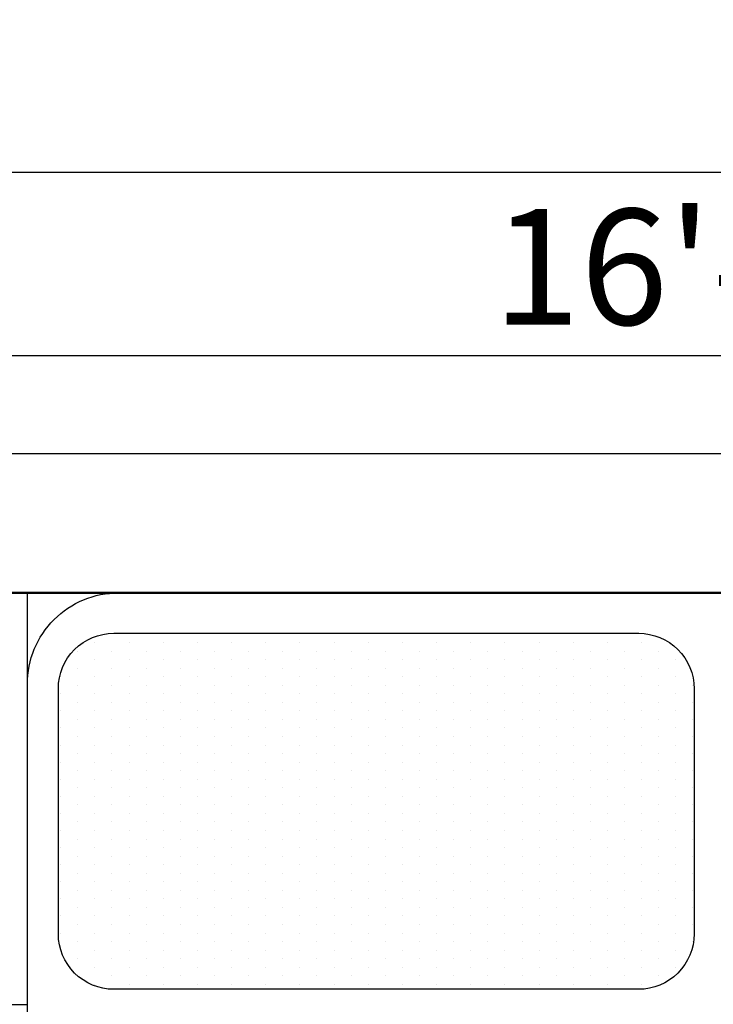
# Model space of a CAD drawing. Units: inches. Extents: x 3064 to 19385, y 846 to 15425.
# Tile 32 of 108: x 4973 to 5003, y 1368 to 1411. Entities that reach past the tile are written whole.
import ezdxf

# ---------------------------------------------------------------- set-up
doc = ezdxf.new("R2010")
doc.units = ezdxf.units.IN
for name, color, linetype, lineweight in [('A-ANNO-DIMS', 2, 'Continuous', 18), ('A-FLOR-FIXT', 9, 'Continuous', 18), ('A-WALL', 7, 'Continuous', 50), ('C-PROP', 6, 'Continuous', 25)]:
    doc.layers.add(name, color=color, linetype=linetype, lineweight=lineweight)
doc.layers.add('BLOCK', color=6, linetype='Continuous')
doc.styles.get("Standard").update_dxf_attribs({"font": 'arial.ttf'})
doc.dimstyles.new('ISO-25', dxfattribs={"dimtxt": 9, "dimasz": 2.5, "dimexe": 1.25, "dimexo": 0.625, "dimtad": 1, "dimdec": 1, "dimlunit": 3, "dimtxsty": 'Standard', "dimcen": 2.5, "dimadec": 0, "dimazin": 0, "dimtfac": 1, "dimtdec": 1, "dimtmove": 0, "dimatfit": 3, "dimfxl": 1, "dimarcsym": 0})

# ---------------------------------------------------------------- blocks, each defined once
blk = doc.blocks.new('*X7')
at = {"color": 0}
for p, q in [((266.25, 456.9375), (266.25, 456.9375)), ((266.4375, 457.03125), (266.4375, 457.03125)), ((266.625, 456.9375), (266.625, 456.9375)), ((266.8125, 457.03125), (266.8125, 457.03125)), ((267, 456.9375), (267, 456.9375)), ((267.1875, 457.03125), (267.1875, 457.03125)), ((267.375, 456.9375), (267.375, 456.9375)), ((267.5625, 457.03125), (267.5625, 457.03125)), ((267.75, 456.9375), (267.75, 456.9375)), ((267.9375, 457.03125), (267.9375, 457.03125)), ((268.125, 456.9375), (268.125, 456.9375)), ((268.3125, 457.03125), (268.3125, 457.03125)), ((268.5, 456.9375), (268.5, 456.9375)), ((268.6875, 457.03125), (268.6875, 457.03125)), ((268.875, 456.9375), (268.875, 456.9375)), ((269.0625, 457.03125), (269.0625, 457.03125)), ((269.25, 456.9375), (269.25, 456.9375)), ((269.4375, 457.03125), (269.4375, 457.03125)), ((269.625, 456.9375), (269.625, 456.9375)), ((269.8125, 457.03125), (269.8125, 457.03125)), ((270, 456.9375), (270, 456.9375)), ((270.1875, 457.03125), (270.1875, 457.03125)), ((270.375, 456.9375), (270.375, 456.9375)), ((270.5625, 457.03125), (270.5625, 457.03125)), ((270.75, 456.9375), (270.75, 456.9375)), ((270.9375, 457.03125), (270.9375, 457.03125)), ((271.125, 456.9375), (271.125, 456.9375)), ((271.3125, 457.03125), (271.3125, 457.03125)), ((271.5, 456.9375), (271.5, 456.9375)), ((271.6875, 457.03125), (271.6875, 457.03125)), ((271.875, 456.9375), (271.875, 456.9375)), ((272.0625, 457.03125), (272.0625, 457.03125)), ((272.25, 456.9375), (272.25, 456.9375)), ((266.0625, 456.84375), (266.0625, 456.84375)), ((266.4375, 456.84375), (266.4375, 456.84375)), ((266.8125, 456.84375), (266.8125, 456.84375)), ((267.1875, 456.84375), (267.1875, 456.84375)), ((267.5625, 456.84375), (267.5625, 456.84375)), ((267.9375, 456.84375), (267.9375, 456.84375)), ((268.3125, 456.84375), (268.3125, 456.84375)), ((268.6875, 456.84375), (268.6875, 456.84375)), ((269.0625, 456.84375), (269.0625, 456.84375)), ((269.4375, 456.84375), (269.4375, 456.84375)), ((269.8125, 456.84375), (269.8125, 456.84375)), ((270.1875, 456.84375), (270.1875, 456.84375)), ((270.5625, 456.84375), (270.5625, 456.84375)), ((270.9375, 456.84375), (270.9375, 456.84375)), ((271.3125, 456.84375), (271.3125, 456.84375)), ((271.6875, 456.84375), (271.6875, 456.84375)), ((272.0625, 456.84375), (272.0625, 456.84375)), ((272.4375, 456.84375), (272.4375, 456.84375)), ((266.25, 456.75), (266.25, 456.75)), ((266.625, 456.75), (266.625, 456.75)), ((267, 456.75), (267, 456.75)), ((267.375, 456.75), (267.375, 456.75)), ((267.75, 456.75), (267.75, 456.75)), ((268.125, 456.75), (268.125, 456.75)), ((268.5, 456.75), (268.5, 456.75)), ((268.875, 456.75), (268.875, 456.75)), ((269.25, 456.75), (269.25, 456.75)), ((269.625, 456.75), (269.625, 456.75)), ((270, 456.75), (270, 456.75)), ((270.375, 456.75), (270.375, 456.75)), ((270.75, 456.75), (270.75, 456.75)), ((271.125, 456.75), (271.125, 456.75)), ((271.5, 456.75), (271.5, 456.75)), ((271.875, 456.75), (271.875, 456.75)), ((272.25, 456.75), (272.25, 456.75)), ((272.625, 456.75), (272.625, 456.75)), ((266.0625, 456.65625), (266.0625, 456.65625)), ((266.4375, 456.65625), (266.4375, 456.65625)), ((266.8125, 456.65625), (266.8125, 456.65625)), ((267.1875, 456.65625), (267.1875, 456.65625)), ((267.5625, 456.65625), (267.5625, 456.65625)), ((267.9375, 456.65625), (267.9375, 456.65625)), ((268.3125, 456.65625), (268.3125, 456.65625)), ((268.6875, 456.65625), (268.6875, 456.65625)), ((269.0625, 456.65625), (269.0625, 456.65625)), ((269.4375, 456.65625), (269.4375, 456.65625)), ((269.8125, 456.65625), (269.8125, 456.65625)), ((270.1875, 456.65625), (270.1875, 456.65625)), ((270.5625, 456.65625), (270.5625, 456.65625)), ((270.9375, 456.65625), (270.9375, 456.65625)), ((271.3125, 456.65625), (271.3125, 456.65625)), ((271.6875, 456.65625), (271.6875, 456.65625)), ((272.0625, 456.65625), (272.0625, 456.65625)), ((272.4375, 456.65625), (272.4375, 456.65625)), ((265.875, 456.5625), (265.875, 456.5625)), ((266.25, 456.5625), (266.25, 456.5625)), ((266.625, 456.5625), (266.625, 456.5625)), ((267, 456.5625), (267, 456.5625)), ((267.375, 456.5625), (267.375, 456.5625)), ((267.75, 456.5625), (267.75, 456.5625)), ((268.125, 456.5625), (268.125, 456.5625)), ((268.5, 456.5625), (268.5, 456.5625)), ((268.875, 456.5625), (268.875, 456.5625)), ((269.25, 456.5625), (269.25, 456.5625)), ((269.625, 456.5625), (269.625, 456.5625)), ((270, 456.5625), (270, 456.5625)), ((270.375, 456.5625), (270.375, 456.5625)), ((270.75, 456.5625), (270.75, 456.5625)), ((271.125, 456.5625), (271.125, 456.5625)), ((271.5, 456.5625), (271.5, 456.5625)), ((271.875, 456.5625), (271.875, 456.5625)), ((272.25, 456.5625), (272.25, 456.5625)), ((272.625, 456.5625), (272.625, 456.5625)), ((266.0625, 456.46875), (266.0625, 456.46875)), ((266.4375, 456.46875), (266.4375, 456.46875)), ((266.8125, 456.46875), (266.8125, 456.46875)), ((267.1875, 456.46875), (267.1875, 456.46875)), ((267.5625, 456.46875), (267.5625, 456.46875)), ((267.9375, 456.46875), (267.9375, 456.46875)), ((268.3125, 456.46875), (268.3125, 456.46875)), ((268.6875, 456.46875), (268.6875, 456.46875)), ((269.0625, 456.46875), (269.0625, 456.46875)), ((269.4375, 456.46875), (269.4375, 456.46875)), ((269.8125, 456.46875), (269.8125, 456.46875)), ((270.1875, 456.46875), (270.1875, 456.46875)), ((270.5625, 456.46875), (270.5625, 456.46875)), ((270.9375, 456.46875), (270.9375, 456.46875)), ((271.3125, 456.46875), (271.3125, 456.46875)), ((271.6875, 456.46875), (271.6875, 456.46875)), ((272.0625, 456.46875), (272.0625, 456.46875)), ((272.4375, 456.46875), (272.4375, 456.46875)), ((272.8125, 456.46875), (272.8125, 456.46875)), ((265.875, 456.375), (265.875, 456.375)), ((266.25, 456.375), (266.25, 456.375)), ((266.625, 456.375), (266.625, 456.375)), ((267, 456.375), (267, 456.375)), ((267.375, 456.375), (267.375, 456.375)), ((267.75, 456.375), (267.75, 456.375)), ((268.125, 456.375), (268.125, 456.375)), ((268.5, 456.375), (268.5, 456.375)), ((268.875, 456.375), (268.875, 456.375)), ((269.25, 456.375), (269.25, 456.375)), ((269.625, 456.375), (269.625, 456.375)), ((270, 456.375), (270, 456.375)), ((270.375, 456.375), (270.375, 456.375)), ((270.75, 456.375), (270.75, 456.375)), ((271.125, 456.375), (271.125, 456.375)), ((271.5, 456.375), (271.5, 456.375)), ((271.875, 456.375), (271.875, 456.375)), ((272.25, 456.375), (272.25, 456.375)), ((272.625, 456.375), (272.625, 456.375)), ((265.875, 456.1875), (265.875, 456.1875)), ((266.0625, 456.28125), (266.0625, 456.28125)), ((266.25, 456.1875), (266.25, 456.1875)), ((266.4375, 456.28125), (266.4375, 456.28125)), ((266.625, 456.1875), (266.625, 456.1875)), ((266.8125, 456.28125), (266.8125, 456.28125)), ((267, 456.1875), (267, 456.1875)), ((267.1875, 456.28125), (267.1875, 456.28125)), ((267.375, 456.1875), (267.375, 456.1875)), ((267.5625, 456.28125), (267.5625, 456.28125)), ((267.75, 456.1875), (267.75, 456.1875)), ((267.9375, 456.28125), (267.9375, 456.28125)), ((268.125, 456.1875), (268.125, 456.1875)), ((268.3125, 456.28125), (268.3125, 456.28125)), ((268.5, 456.1875), (268.5, 456.1875)), ((268.6875, 456.28125), (268.6875, 456.28125)), ((268.875, 456.1875), (268.875, 456.1875)), ((269.0625, 456.28125), (269.0625, 456.28125)), ((269.25, 456.1875), (269.25, 456.1875)), ((269.4375, 456.28125), (269.4375, 456.28125)), ((269.625, 456.1875), (269.625, 456.1875)), ((269.8125, 456.28125), (269.8125, 456.28125)), ((270, 456.1875), (270, 456.1875)), ((270.1875, 456.28125), (270.1875, 456.28125)), ((270.375, 456.1875), (270.375, 456.1875)), ((270.5625, 456.28125), (270.5625, 456.28125)), ((270.75, 456.1875), (270.75, 456.1875)), ((270.9375, 456.28125), (270.9375, 456.28125)), ((271.125, 456.1875), (271.125, 456.1875)), ((271.3125, 456.28125), (271.3125, 456.28125)), ((271.5, 456.1875), (271.5, 456.1875)), ((271.6875, 456.28125), (271.6875, 456.28125)), ((271.875, 456.1875), (271.875, 456.1875)), ((272.0625, 456.28125), (272.0625, 456.28125)), ((272.25, 456.1875), (272.25, 456.1875)), ((272.4375, 456.28125), (272.4375, 456.28125)), ((272.625, 456.1875), (272.625, 456.1875)), ((272.8125, 456.28125), (272.8125, 456.28125)), ((266.0625, 456.09375), (266.0625, 456.09375)), ((266.4375, 456.09375), (266.4375, 456.09375)), ((266.8125, 456.09375), (266.8125, 456.09375)), ((267.1875, 456.09375), (267.1875, 456.09375)), ((267.5625, 456.09375), (267.5625, 456.09375)), ((267.9375, 456.09375), (267.9375, 456.09375)), ((268.3125, 456.09375), (268.3125, 456.09375)), ((268.6875, 456.09375), (268.6875, 456.09375)), ((269.0625, 456.09375), (269.0625, 456.09375)), ((269.4375, 456.09375), (269.4375, 456.09375)), ((269.8125, 456.09375), (269.8125, 456.09375)), ((270.1875, 456.09375), (270.1875, 456.09375)), ((270.5625, 456.09375), (270.5625, 456.09375)), ((270.9375, 456.09375), (270.9375, 456.09375)), ((271.3125, 456.09375), (271.3125, 456.09375)), ((271.6875, 456.09375), (271.6875, 456.09375)), ((272.0625, 456.09375), (272.0625, 456.09375)), ((272.4375, 456.09375), (272.4375, 456.09375)), ((272.8125, 456.09375), (272.8125, 456.09375)), ((265.875, 456), (265.875, 456)), ((266.25, 456), (266.25, 456)), ((266.625, 456), (266.625, 456)), ((267, 456), (267, 456)), ((267.375, 456), (267.375, 456)), ((267.75, 456), (267.75, 456)), ((268.125, 456), (268.125, 456)), ((268.5, 456), (268.5, 456)), ((268.875, 456), (268.875, 456)), ((269.25, 456), (269.25, 456)), ((269.625, 456), (269.625, 456)), ((270, 456), (270, 456)), ((270.375, 456), (270.375, 456)), ((270.75, 456), (270.75, 456)), ((271.125, 456), (271.125, 456)), ((271.5, 456), (271.5, 456)), ((271.875, 456), (271.875, 456)), ((272.25, 456), (272.25, 456)), ((272.625, 456), (272.625, 456)), ((266.0625, 455.90625), (266.0625, 455.90625)), ((266.4375, 455.90625), (266.4375, 455.90625)), ((266.8125, 455.90625), (266.8125, 455.90625)), ((267.1875, 455.90625), (267.1875, 455.90625)), ((267.5625, 455.90625), (267.5625, 455.90625)), ((267.9375, 455.90625), (267.9375, 455.90625)), ((268.3125, 455.90625), (268.3125, 455.90625)), ((268.6875, 455.90625), (268.6875, 455.90625)), ((269.0625, 455.90625), (269.0625, 455.90625)), ((269.4375, 455.90625), (269.4375, 455.90625)), ((269.8125, 455.90625), (269.8125, 455.90625)), ((270.1875, 455.90625), (270.1875, 455.90625)), ((270.5625, 455.90625), (270.5625, 455.90625)), ((270.9375, 455.90625), (270.9375, 455.90625)), ((271.3125, 455.90625), (271.3125, 455.90625)), ((271.6875, 455.90625), (271.6875, 455.90625)), ((272.0625, 455.90625), (272.0625, 455.90625)), ((272.4375, 455.90625), (272.4375, 455.90625)), ((272.8125, 455.90625), (272.8125, 455.90625)), ((265.875, 455.8125), (265.875, 455.8125)), ((266.25, 455.8125), (266.25, 455.8125)), ((266.625, 455.8125), (266.625, 455.8125)), ((267, 455.8125), (267, 455.8125)), ((267.375, 455.8125), (267.375, 455.8125)), ((267.75, 455.8125), (267.75, 455.8125)), ((268.125, 455.8125), (268.125, 455.8125)), ((268.5, 455.8125), (268.5, 455.8125)), ((268.875, 455.8125), (268.875, 455.8125)), ((269.25, 455.8125), (269.25, 455.8125)), ((269.625, 455.8125), (269.625, 455.8125)), ((270, 455.8125), (270, 455.8125)), ((270.375, 455.8125), (270.375, 455.8125)), ((270.75, 455.8125), (270.75, 455.8125)), ((271.125, 455.8125), (271.125, 455.8125)), ((271.5, 455.8125), (271.5, 455.8125)), ((271.875, 455.8125), (271.875, 455.8125)), ((272.25, 455.8125), (272.25, 455.8125)), ((272.625, 455.8125), (272.625, 455.8125)), ((266.0625, 455.71875), (266.0625, 455.71875)), ((266.4375, 455.71875), (266.4375, 455.71875)), ((266.8125, 455.71875), (266.8125, 455.71875)), ((267.1875, 455.71875), (267.1875, 455.71875)), ((267.5625, 455.71875), (267.5625, 455.71875)), ((267.9375, 455.71875), (267.9375, 455.71875)), ((268.3125, 455.71875), (268.3125, 455.71875)), ((268.6875, 455.71875), (268.6875, 455.71875)), ((269.0625, 455.71875), (269.0625, 455.71875)), ((269.4375, 455.71875), (269.4375, 455.71875)), ((269.8125, 455.71875), (269.8125, 455.71875)), ((270.1875, 455.71875), (270.1875, 455.71875)), ((270.5625, 455.71875), (270.5625, 455.71875)), ((270.9375, 455.71875), (270.9375, 455.71875)), ((271.3125, 455.71875), (271.3125, 455.71875)), ((271.6875, 455.71875), (271.6875, 455.71875)), ((272.0625, 455.71875), (272.0625, 455.71875)), ((272.4375, 455.71875), (272.4375, 455.71875)), ((272.8125, 455.71875), (272.8125, 455.71875)), ((265.875, 455.625), (265.875, 455.625)), ((266.0625, 455.53125), (266.0625, 455.53125)), ((266.25, 455.625), (266.25, 455.625)), ((266.4375, 455.53125), (266.4375, 455.53125)), ((266.625, 455.625), (266.625, 455.625)), ((266.8125, 455.53125), (266.8125, 455.53125)), ((267, 455.625), (267, 455.625)), ((267.1875, 455.53125), (267.1875, 455.53125)), ((267.375, 455.625), (267.375, 455.625)), ((267.5625, 455.53125), (267.5625, 455.53125)), ((267.75, 455.625), (267.75, 455.625)), ((267.9375, 455.53125), (267.9375, 455.53125)), ((268.125, 455.625), (268.125, 455.625)), ((268.3125, 455.53125), (268.3125, 455.53125)), ((268.5, 455.625), (268.5, 455.625)), ((268.6875, 455.53125), (268.6875, 455.53125)), ((268.875, 455.625), (268.875, 455.625)), ((269.0625, 455.53125), (269.0625, 455.53125)), ((269.25, 455.625), (269.25, 455.625)), ((269.4375, 455.53125), (269.4375, 455.53125)), ((269.625, 455.625), (269.625, 455.625)), ((269.8125, 455.53125), (269.8125, 455.53125)), ((270, 455.625), (270, 455.625)), ((270.1875, 455.53125), (270.1875, 455.53125)), ((270.375, 455.625), (270.375, 455.625)), ((270.5625, 455.53125), (270.5625, 455.53125)), ((270.75, 455.625), (270.75, 455.625)), ((270.9375, 455.53125), (270.9375, 455.53125)), ((271.125, 455.625), (271.125, 455.625)), ((271.3125, 455.53125), (271.3125, 455.53125)), ((271.5, 455.625), (271.5, 455.625)), ((271.6875, 455.53125), (271.6875, 455.53125)), ((271.875, 455.625), (271.875, 455.625)), ((272.0625, 455.53125), (272.0625, 455.53125)), ((272.25, 455.625), (272.25, 455.625)), ((272.4375, 455.53125), (272.4375, 455.53125)), ((272.625, 455.625), (272.625, 455.625)), ((272.8125, 455.53125), (272.8125, 455.53125)), ((265.875, 455.4375), (265.875, 455.4375)), ((266.25, 455.4375), (266.25, 455.4375)), ((266.625, 455.4375), (266.625, 455.4375)), ((267, 455.4375), (267, 455.4375)), ((267.375, 455.4375), (267.375, 455.4375)), ((267.75, 455.4375), (267.75, 455.4375)), ((268.125, 455.4375), (268.125, 455.4375)), ((268.5, 455.4375), (268.5, 455.4375)), ((268.875, 455.4375), (268.875, 455.4375)), ((269.25, 455.4375), (269.25, 455.4375)), ((269.625, 455.4375), (269.625, 455.4375)), ((270, 455.4375), (270, 455.4375)), ((270.375, 455.4375), (270.375, 455.4375)), ((270.75, 455.4375), (270.75, 455.4375)), ((271.125, 455.4375), (271.125, 455.4375)), ((271.5, 455.4375), (271.5, 455.4375)), ((271.875, 455.4375), (271.875, 455.4375)), ((272.25, 455.4375), (272.25, 455.4375)), ((272.625, 455.4375), (272.625, 455.4375)), ((266.0625, 455.34375), (266.0625, 455.34375)), ((266.4375, 455.34375), (266.4375, 455.34375)), ((266.8125, 455.34375), (266.8125, 455.34375)), ((267.1875, 455.34375), (267.1875, 455.34375)), ((267.5625, 455.34375), (267.5625, 455.34375)), ((267.9375, 455.34375), (267.9375, 455.34375)), ((268.3125, 455.34375), (268.3125, 455.34375)), ((268.6875, 455.34375), (268.6875, 455.34375)), ((269.0625, 455.34375), (269.0625, 455.34375)), ((269.4375, 455.34375), (269.4375, 455.34375)), ((269.8125, 455.34375), (269.8125, 455.34375)), ((270.1875, 455.34375), (270.1875, 455.34375)), ((270.5625, 455.34375), (270.5625, 455.34375)), ((270.9375, 455.34375), (270.9375, 455.34375)), ((271.3125, 455.34375), (271.3125, 455.34375)), ((271.6875, 455.34375), (271.6875, 455.34375)), ((272.0625, 455.34375), (272.0625, 455.34375)), ((272.4375, 455.34375), (272.4375, 455.34375)), ((272.8125, 455.34375), (272.8125, 455.34375)), ((265.875, 455.25), (265.875, 455.25)), ((266.25, 455.25), (266.25, 455.25)), ((266.625, 455.25), (266.625, 455.25)), ((267, 455.25), (267, 455.25)), ((267.375, 455.25), (267.375, 455.25)), ((267.75, 455.25), (267.75, 455.25)), ((268.125, 455.25), (268.125, 455.25)), ((268.5, 455.25), (268.5, 455.25)), ((268.875, 455.25), (268.875, 455.25)), ((269.25, 455.25), (269.25, 455.25)), ((269.625, 455.25), (269.625, 455.25)), ((270, 455.25), (270, 455.25)), ((270.375, 455.25), (270.375, 455.25)), ((270.75, 455.25), (270.75, 455.25)), ((271.125, 455.25), (271.125, 455.25)), ((271.5, 455.25), (271.5, 455.25)), ((271.875, 455.25), (271.875, 455.25)), ((272.25, 455.25), (272.25, 455.25)), ((272.625, 455.25), (272.625, 455.25)), ((266.0625, 455.15625), (266.0625, 455.15625)), ((266.4375, 455.15625), (266.4375, 455.15625)), ((266.8125, 455.15625), (266.8125, 455.15625)), ((267.1875, 455.15625), (267.1875, 455.15625)), ((267.5625, 455.15625), (267.5625, 455.15625)), ((267.9375, 455.15625), (267.9375, 455.15625)), ((268.3125, 455.15625), (268.3125, 455.15625)), ((268.6875, 455.15625), (268.6875, 455.15625)), ((269.0625, 455.15625), (269.0625, 455.15625)), ((269.4375, 455.15625), (269.4375, 455.15625)), ((269.8125, 455.15625), (269.8125, 455.15625)), ((270.1875, 455.15625), (270.1875, 455.15625)), ((270.5625, 455.15625), (270.5625, 455.15625)), ((270.9375, 455.15625), (270.9375, 455.15625)), ((271.3125, 455.15625), (271.3125, 455.15625)), ((271.6875, 455.15625), (271.6875, 455.15625)), ((272.0625, 455.15625), (272.0625, 455.15625)), ((272.4375, 455.15625), (272.4375, 455.15625)), ((272.8125, 455.15625), (272.8125, 455.15625)), ((265.875, 455.0625), (265.875, 455.0625)), ((266.25, 455.0625), (266.25, 455.0625)), ((266.625, 455.0625), (266.625, 455.0625)), ((267, 455.0625), (267, 455.0625)), ((267.375, 455.0625), (267.375, 455.0625)), ((267.75, 455.0625), (267.75, 455.0625)), ((268.125, 455.0625), (268.125, 455.0625)), ((268.5, 455.0625), (268.5, 455.0625)), ((268.875, 455.0625), (268.875, 455.0625)), ((269.25, 455.0625), (269.25, 455.0625)), ((269.625, 455.0625), (269.625, 455.0625)), ((270, 455.0625), (270, 455.0625)), ((270.375, 455.0625), (270.375, 455.0625)), ((270.75, 455.0625), (270.75, 455.0625)), ((271.125, 455.0625), (271.125, 455.0625)), ((271.5, 455.0625), (271.5, 455.0625)), ((271.875, 455.0625), (271.875, 455.0625)), ((272.25, 455.0625), (272.25, 455.0625)), ((272.625, 455.0625), (272.625, 455.0625)), ((266.0625, 454.96875), (266.0625, 454.96875)), ((266.4375, 454.96875), (266.4375, 454.96875)), ((266.8125, 454.96875), (266.8125, 454.96875)), ((267.1875, 454.96875), (267.1875, 454.96875)), ((267.5625, 454.96875), (267.5625, 454.96875)), ((267.9375, 454.96875), (267.9375, 454.96875)), ((268.3125, 454.96875), (268.3125, 454.96875)), ((268.6875, 454.96875), (268.6875, 454.96875)), ((269.0625, 454.96875), (269.0625, 454.96875)), ((269.4375, 454.96875), (269.4375, 454.96875)), ((269.8125, 454.96875), (269.8125, 454.96875)), ((270.1875, 454.96875), (270.1875, 454.96875)), ((270.5625, 454.96875), (270.5625, 454.96875)), ((270.9375, 454.96875), (270.9375, 454.96875)), ((271.3125, 454.96875), (271.3125, 454.96875)), ((271.6875, 454.96875), (271.6875, 454.96875)), ((272.0625, 454.96875), (272.0625, 454.96875)), ((272.4375, 454.96875), (272.4375, 454.96875)), ((272.8125, 454.96875), (272.8125, 454.96875)), ((265.875, 454.875), (265.875, 454.875)), ((266.0625, 454.78125), (266.0625, 454.78125)), ((266.25, 454.875), (266.25, 454.875)), ((266.4375, 454.78125), (266.4375, 454.78125)), ((266.625, 454.875), (266.625, 454.875)), ((266.8125, 454.78125), (266.8125, 454.78125)), ((267, 454.875), (267, 454.875)), ((267.1875, 454.78125), (267.1875, 454.78125)), ((267.375, 454.875), (267.375, 454.875)), ((267.5625, 454.78125), (267.5625, 454.78125)), ((267.75, 454.875), (267.75, 454.875)), ((267.9375, 454.78125), (267.9375, 454.78125)), ((268.125, 454.875), (268.125, 454.875)), ((268.3125, 454.78125), (268.3125, 454.78125)), ((268.5, 454.875), (268.5, 454.875)), ((268.6875, 454.78125), (268.6875, 454.78125)), ((268.875, 454.875), (268.875, 454.875)), ((269.0625, 454.78125), (269.0625, 454.78125)), ((269.25, 454.875), (269.25, 454.875)), ((269.4375, 454.78125), (269.4375, 454.78125)), ((269.625, 454.875), (269.625, 454.875)), ((269.8125, 454.78125), (269.8125, 454.78125)), ((270, 454.875), (270, 454.875)), ((270.1875, 454.78125), (270.1875, 454.78125)), ((270.375, 454.875), (270.375, 454.875)), ((270.5625, 454.78125), (270.5625, 454.78125)), ((270.75, 454.875), (270.75, 454.875)), ((270.9375, 454.78125), (270.9375, 454.78125)), ((271.125, 454.875), (271.125, 454.875)), ((271.3125, 454.78125), (271.3125, 454.78125)), ((271.5, 454.875), (271.5, 454.875)), ((271.6875, 454.78125), (271.6875, 454.78125)), ((271.875, 454.875), (271.875, 454.875)), ((272.0625, 454.78125), (272.0625, 454.78125)), ((272.25, 454.875), (272.25, 454.875)), ((272.4375, 454.78125), (272.4375, 454.78125)), ((272.625, 454.875), (272.625, 454.875)), ((272.8125, 454.78125), (272.8125, 454.78125)), ((265.875, 454.6875), (265.875, 454.6875)), ((266.25, 454.6875), (266.25, 454.6875)), ((266.625, 454.6875), (266.625, 454.6875)), ((267, 454.6875), (267, 454.6875)), ((267.375, 454.6875), (267.375, 454.6875)), ((267.75, 454.6875), (267.75, 454.6875)), ((268.125, 454.6875), (268.125, 454.6875)), ((268.5, 454.6875), (268.5, 454.6875)), ((268.875, 454.6875), (268.875, 454.6875)), ((269.25, 454.6875), (269.25, 454.6875)), ((269.625, 454.6875), (269.625, 454.6875)), ((270, 454.6875), (270, 454.6875)), ((270.375, 454.6875), (270.375, 454.6875)), ((270.75, 454.6875), (270.75, 454.6875)), ((271.125, 454.6875), (271.125, 454.6875)), ((271.5, 454.6875), (271.5, 454.6875)), ((271.875, 454.6875), (271.875, 454.6875)), ((272.25, 454.6875), (272.25, 454.6875)), ((272.625, 454.6875), (272.625, 454.6875)), ((266.0625, 454.59375), (266.0625, 454.59375)), ((266.4375, 454.59375), (266.4375, 454.59375)), ((266.8125, 454.59375), (266.8125, 454.59375)), ((267.1875, 454.59375), (267.1875, 454.59375)), ((267.5625, 454.59375), (267.5625, 454.59375)), ((267.9375, 454.59375), (267.9375, 454.59375)), ((268.3125, 454.59375), (268.3125, 454.59375)), ((268.6875, 454.59375), (268.6875, 454.59375)), ((269.0625, 454.59375), (269.0625, 454.59375)), ((269.4375, 454.59375), (269.4375, 454.59375)), ((269.8125, 454.59375), (269.8125, 454.59375)), ((270.1875, 454.59375), (270.1875, 454.59375)), ((270.5625, 454.59375), (270.5625, 454.59375)), ((270.9375, 454.59375), (270.9375, 454.59375)), ((271.3125, 454.59375), (271.3125, 454.59375)), ((271.6875, 454.59375), (271.6875, 454.59375)), ((272.0625, 454.59375), (272.0625, 454.59375)), ((272.4375, 454.59375), (272.4375, 454.59375)), ((272.8125, 454.59375), (272.8125, 454.59375)), ((265.875, 454.5), (265.875, 454.5)), ((266.25, 454.5), (266.25, 454.5)), ((266.625, 454.5), (266.625, 454.5)), ((267, 454.5), (267, 454.5)), ((267.375, 454.5), (267.375, 454.5)), ((267.75, 454.5), (267.75, 454.5)), ((268.125, 454.5), (268.125, 454.5)), ((268.5, 454.5), (268.5, 454.5)), ((268.875, 454.5), (268.875, 454.5)), ((269.25, 454.5), (269.25, 454.5)), ((269.625, 454.5), (269.625, 454.5)), ((270, 454.5), (270, 454.5)), ((270.375, 454.5), (270.375, 454.5)), ((270.75, 454.5), (270.75, 454.5)), ((271.125, 454.5), (271.125, 454.5)), ((271.5, 454.5), (271.5, 454.5)), ((271.875, 454.5), (271.875, 454.5)), ((272.25, 454.5), (272.25, 454.5)), ((272.625, 454.5), (272.625, 454.5)), ((266.0625, 454.40625), (266.0625, 454.40625)), ((266.4375, 454.40625), (266.4375, 454.40625)), ((266.8125, 454.40625), (266.8125, 454.40625)), ((267.1875, 454.40625), (267.1875, 454.40625)), ((267.5625, 454.40625), (267.5625, 454.40625)), ((267.9375, 454.40625), (267.9375, 454.40625)), ((268.3125, 454.40625), (268.3125, 454.40625)), ((268.6875, 454.40625), (268.6875, 454.40625)), ((269.0625, 454.40625), (269.0625, 454.40625)), ((269.4375, 454.40625), (269.4375, 454.40625)), ((269.8125, 454.40625), (269.8125, 454.40625)), ((270.1875, 454.40625), (270.1875, 454.40625)), ((270.5625, 454.40625), (270.5625, 454.40625)), ((270.9375, 454.40625), (270.9375, 454.40625)), ((271.3125, 454.40625), (271.3125, 454.40625)), ((271.6875, 454.40625), (271.6875, 454.40625)), ((272.0625, 454.40625), (272.0625, 454.40625)), ((272.4375, 454.40625), (272.4375, 454.40625)), ((272.8125, 454.40625), (272.8125, 454.40625)), ((265.875, 454.3125), (265.875, 454.3125)), ((266.25, 454.3125), (266.25, 454.3125)), ((266.625, 454.3125), (266.625, 454.3125)), ((267, 454.3125), (267, 454.3125)), ((267.375, 454.3125), (267.375, 454.3125)), ((267.75, 454.3125), (267.75, 454.3125)), ((268.125, 454.3125), (268.125, 454.3125)), ((268.5, 454.3125), (268.5, 454.3125)), ((268.875, 454.3125), (268.875, 454.3125)), ((269.25, 454.3125), (269.25, 454.3125)), ((269.625, 454.3125), (269.625, 454.3125)), ((270, 454.3125), (270, 454.3125)), ((270.375, 454.3125), (270.375, 454.3125)), ((270.75, 454.3125), (270.75, 454.3125)), ((271.125, 454.3125), (271.125, 454.3125)), ((271.5, 454.3125), (271.5, 454.3125)), ((271.875, 454.3125), (271.875, 454.3125)), ((272.25, 454.3125), (272.25, 454.3125)), ((272.625, 454.3125), (272.625, 454.3125)), ((266.0625, 454.21875), (266.0625, 454.21875)), ((266.4375, 454.21875), (266.4375, 454.21875)), ((266.8125, 454.21875), (266.8125, 454.21875)), ((267.1875, 454.21875), (267.1875, 454.21875)), ((267.5625, 454.21875), (267.5625, 454.21875)), ((267.9375, 454.21875), (267.9375, 454.21875)), ((268.3125, 454.21875), (268.3125, 454.21875)), ((268.6875, 454.21875), (268.6875, 454.21875)), ((269.0625, 454.21875), (269.0625, 454.21875)), ((269.4375, 454.21875), (269.4375, 454.21875)), ((269.8125, 454.21875), (269.8125, 454.21875)), ((270.1875, 454.21875), (270.1875, 454.21875)), ((270.5625, 454.21875), (270.5625, 454.21875)), ((270.9375, 454.21875), (270.9375, 454.21875)), ((271.3125, 454.21875), (271.3125, 454.21875)), ((271.6875, 454.21875), (271.6875, 454.21875)), ((272.0625, 454.21875), (272.0625, 454.21875)), ((272.4375, 454.21875), (272.4375, 454.21875)), ((272.8125, 454.21875), (272.8125, 454.21875)), ((265.875, 454.125), (265.875, 454.125)), ((266.0625, 454.03125), (266.0625, 454.03125)), ((266.25, 454.125), (266.25, 454.125)), ((266.4375, 454.03125), (266.4375, 454.03125)), ((266.625, 454.125), (266.625, 454.125)), ((266.8125, 454.03125), (266.8125, 454.03125)), ((267, 454.125), (267, 454.125)), ((267.1875, 454.03125), (267.1875, 454.03125)), ((267.375, 454.125), (267.375, 454.125)), ((267.5625, 454.03125), (267.5625, 454.03125)), ((267.75, 454.125), (267.75, 454.125)), ((267.9375, 454.03125), (267.9375, 454.03125)), ((268.125, 454.125), (268.125, 454.125)), ((268.3125, 454.03125), (268.3125, 454.03125)), ((268.5, 454.125), (268.5, 454.125)), ((268.6875, 454.03125), (268.6875, 454.03125)), ((268.875, 454.125), (268.875, 454.125)), ((269.0625, 454.03125), (269.0625, 454.03125)), ((269.25, 454.125), (269.25, 454.125)), ((269.4375, 454.03125), (269.4375, 454.03125)), ((269.625, 454.125), (269.625, 454.125)), ((269.8125, 454.03125), (269.8125, 454.03125)), ((270, 454.125), (270, 454.125)), ((270.1875, 454.03125), (270.1875, 454.03125)), ((270.375, 454.125), (270.375, 454.125)), ((270.5625, 454.03125), (270.5625, 454.03125)), ((270.75, 454.125), (270.75, 454.125)), ((270.9375, 454.03125), (270.9375, 454.03125)), ((271.125, 454.125), (271.125, 454.125)), ((271.3125, 454.03125), (271.3125, 454.03125)), ((271.5, 454.125), (271.5, 454.125)), ((271.6875, 454.03125), (271.6875, 454.03125)), ((271.875, 454.125), (271.875, 454.125)), ((272.0625, 454.03125), (272.0625, 454.03125)), ((272.25, 454.125), (272.25, 454.125)), ((272.4375, 454.03125), (272.4375, 454.03125)), ((272.625, 454.125), (272.625, 454.125)), ((272.8125, 454.03125), (272.8125, 454.03125)), ((265.875, 453.9375), (265.875, 453.9375)), ((266.25, 453.9375), (266.25, 453.9375)), ((266.625, 453.9375), (266.625, 453.9375)), ((267, 453.9375), (267, 453.9375)), ((267.375, 453.9375), (267.375, 453.9375)), ((267.75, 453.9375), (267.75, 453.9375)), ((268.125, 453.9375), (268.125, 453.9375)), ((268.5, 453.9375), (268.5, 453.9375)), ((268.875, 453.9375), (268.875, 453.9375)), ((269.25, 453.9375), (269.25, 453.9375)), ((269.625, 453.9375), (269.625, 453.9375)), ((270, 453.9375), (270, 453.9375)), ((270.375, 453.9375), (270.375, 453.9375)), ((270.75, 453.9375), (270.75, 453.9375)), ((271.125, 453.9375), (271.125, 453.9375)), ((271.5, 453.9375), (271.5, 453.9375)), ((271.875, 453.9375), (271.875, 453.9375)), ((272.25, 453.9375), (272.25, 453.9375)), ((272.625, 453.9375), (272.625, 453.9375)), ((266.0625, 453.84375), (266.0625, 453.84375)), ((266.4375, 453.84375), (266.4375, 453.84375)), ((266.8125, 453.84375), (266.8125, 453.84375)), ((267.1875, 453.84375), (267.1875, 453.84375)), ((267.5625, 453.84375), (267.5625, 453.84375)), ((267.9375, 453.84375), (267.9375, 453.84375)), ((268.3125, 453.84375), (268.3125, 453.84375)), ((268.6875, 453.84375), (268.6875, 453.84375)), ((269.0625, 453.84375), (269.0625, 453.84375)), ((269.4375, 453.84375), (269.4375, 453.84375)), ((269.8125, 453.84375), (269.8125, 453.84375)), ((270.1875, 453.84375), (270.1875, 453.84375)), ((270.5625, 453.84375), (270.5625, 453.84375)), ((270.9375, 453.84375), (270.9375, 453.84375)), ((271.3125, 453.84375), (271.3125, 453.84375)), ((271.6875, 453.84375), (271.6875, 453.84375)), ((272.0625, 453.84375), (272.0625, 453.84375)), ((272.4375, 453.84375), (272.4375, 453.84375)), ((272.8125, 453.84375), (272.8125, 453.84375)), ((265.875, 453.75), (265.875, 453.75)), ((266.25, 453.75), (266.25, 453.75)), ((266.625, 453.75), (266.625, 453.75)), ((267, 453.75), (267, 453.75)), ((267.375, 453.75), (267.375, 453.75)), ((267.75, 453.75), (267.75, 453.75)), ((268.125, 453.75), (268.125, 453.75)), ((268.5, 453.75), (268.5, 453.75)), ((268.875, 453.75), (268.875, 453.75)), ((269.25, 453.75), (269.25, 453.75)), ((269.625, 453.75), (269.625, 453.75)), ((270, 453.75), (270, 453.75)), ((270.375, 453.75), (270.375, 453.75)), ((270.75, 453.75), (270.75, 453.75)), ((271.125, 453.75), (271.125, 453.75)), ((271.5, 453.75), (271.5, 453.75)), ((271.875, 453.75), (271.875, 453.75)), ((272.25, 453.75), (272.25, 453.75)), ((272.625, 453.75), (272.625, 453.75)), ((266.0625, 453.65625), (266.0625, 453.65625)), ((266.4375, 453.65625), (266.4375, 453.65625)), ((266.8125, 453.65625), (266.8125, 453.65625)), ((267.1875, 453.65625), (267.1875, 453.65625)), ((267.5625, 453.65625), (267.5625, 453.65625)), ((267.9375, 453.65625), (267.9375, 453.65625)), ((268.3125, 453.65625), (268.3125, 453.65625)), ((268.6875, 453.65625), (268.6875, 453.65625)), ((269.0625, 453.65625), (269.0625, 453.65625)), ((269.4375, 453.65625), (269.4375, 453.65625)), ((269.8125, 453.65625), (269.8125, 453.65625)), ((270.1875, 453.65625), (270.1875, 453.65625)), ((270.5625, 453.65625), (270.5625, 453.65625)), ((270.9375, 453.65625), (270.9375, 453.65625)), ((271.3125, 453.65625), (271.3125, 453.65625)), ((271.6875, 453.65625), (271.6875, 453.65625)), ((272.0625, 453.65625), (272.0625, 453.65625)), ((272.4375, 453.65625), (272.4375, 453.65625)), ((272.8125, 453.65625), (272.8125, 453.65625)), ((266.25, 453.5625), (266.25, 453.5625)), ((266.625, 453.5625), (266.625, 453.5625)), ((267, 453.5625), (267, 453.5625)), ((267.375, 453.5625), (267.375, 453.5625)), ((267.75, 453.5625), (267.75, 453.5625)), ((268.125, 453.5625), (268.125, 453.5625)), ((268.5, 453.5625), (268.5, 453.5625)), ((268.875, 453.5625), (268.875, 453.5625)), ((269.25, 453.5625), (269.25, 453.5625)), ((269.625, 453.5625), (269.625, 453.5625)), ((270, 453.5625), (270, 453.5625)), ((270.375, 453.5625), (270.375, 453.5625)), ((270.75, 453.5625), (270.75, 453.5625)), ((271.125, 453.5625), (271.125, 453.5625)), ((271.5, 453.5625), (271.5, 453.5625)), ((271.875, 453.5625), (271.875, 453.5625)), ((272.25, 453.5625), (272.25, 453.5625)), ((272.625, 453.5625), (272.625, 453.5625)), ((266.0625, 453.46875), (266.0625, 453.46875)), ((266.25, 453.375), (266.25, 453.375)), ((266.4375, 453.46875), (266.4375, 453.46875)), ((266.625, 453.375), (266.625, 453.375)), ((266.8125, 453.46875), (266.8125, 453.46875)), ((267, 453.375), (267, 453.375)), ((267.1875, 453.46875), (267.1875, 453.46875)), ((267.375, 453.375), (267.375, 453.375)), ((267.5625, 453.46875), (267.5625, 453.46875)), ((267.75, 453.375), (267.75, 453.375)), ((267.9375, 453.46875), (267.9375, 453.46875)), ((268.125, 453.375), (268.125, 453.375)), ((268.3125, 453.46875), (268.3125, 453.46875)), ((268.5, 453.375), (268.5, 453.375)), ((268.6875, 453.46875), (268.6875, 453.46875)), ((268.875, 453.375), (268.875, 453.375)), ((269.0625, 453.46875), (269.0625, 453.46875)), ((269.25, 453.375), (269.25, 453.375)), ((269.4375, 453.46875), (269.4375, 453.46875)), ((269.625, 453.375), (269.625, 453.375)), ((269.8125, 453.46875), (269.8125, 453.46875)), ((270, 453.375), (270, 453.375)), ((270.1875, 453.46875), (270.1875, 453.46875)), ((270.375, 453.375), (270.375, 453.375)), ((270.5625, 453.46875), (270.5625, 453.46875)), ((270.75, 453.375), (270.75, 453.375)), ((270.9375, 453.46875), (270.9375, 453.46875)), ((271.125, 453.375), (271.125, 453.375)), ((271.3125, 453.46875), (271.3125, 453.46875)), ((271.5, 453.375), (271.5, 453.375)), ((271.6875, 453.46875), (271.6875, 453.46875)), ((271.875, 453.375), (271.875, 453.375)), ((272.0625, 453.46875), (272.0625, 453.46875)), ((272.25, 453.375), (272.25, 453.375)), ((272.4375, 453.46875), (272.4375, 453.46875)), ((272.625, 453.375), (272.625, 453.375)), ((266.0625, 453.28125), (266.0625, 453.28125)), ((266.4375, 453.28125), (266.4375, 453.28125)), ((266.8125, 453.28125), (266.8125, 453.28125)), ((267.1875, 453.28125), (267.1875, 453.28125)), ((267.5625, 453.28125), (267.5625, 453.28125)), ((267.9375, 453.28125), (267.9375, 453.28125)), ((268.3125, 453.28125), (268.3125, 453.28125)), ((268.6875, 453.28125), (268.6875, 453.28125)), ((269.0625, 453.28125), (269.0625, 453.28125)), ((269.4375, 453.28125), (269.4375, 453.28125)), ((269.8125, 453.28125), (269.8125, 453.28125)), ((270.1875, 453.28125), (270.1875, 453.28125)), ((270.5625, 453.28125), (270.5625, 453.28125)), ((270.9375, 453.28125), (270.9375, 453.28125)), ((271.3125, 453.28125), (271.3125, 453.28125)), ((271.6875, 453.28125), (271.6875, 453.28125)), ((272.0625, 453.28125), (272.0625, 453.28125)), ((272.4375, 453.28125), (272.4375, 453.28125)), ((266.25, 453.1875), (266.25, 453.1875)), ((266.625, 453.1875), (266.625, 453.1875)), ((267, 453.1875), (267, 453.1875)), ((267.375, 453.1875), (267.375, 453.1875)), ((267.75, 453.1875), (267.75, 453.1875)), ((268.125, 453.1875), (268.125, 453.1875)), ((268.5, 453.1875), (268.5, 453.1875)), ((268.875, 453.1875), (268.875, 453.1875)), ((269.25, 453.1875), (269.25, 453.1875)), ((269.625, 453.1875), (269.625, 453.1875)), ((270, 453.1875), (270, 453.1875)), ((270.375, 453.1875), (270.375, 453.1875)), ((270.75, 453.1875), (270.75, 453.1875)), ((271.125, 453.1875), (271.125, 453.1875)), ((271.5, 453.1875), (271.5, 453.1875)), ((271.875, 453.1875), (271.875, 453.1875)), ((272.25, 453.1875), (272.25, 453.1875))]:
    blk.add_line(p, q, dxfattribs=at)
blk = doc.blocks.new('A$C52E67D0D')
at = {"layer": 'BLOCK'}
blk.add_lwpolyline([(501, 1348.6), (501, 1799.6), (0, 1799.6), (0, 1348.6)], close=True, dxfattribs=at)
for points in [[(1901, 0), (601, 0, -0.414214), (501, 100), (501, 1700, -0.414214), (601, 1800), (1901, 1800, -0.414214), (2001, 1700), (2001, 100, -0.414214)], [(1171.8, 1365.1), (595.8, 1365.1, -0.414214), (535, 1425.9), (535, 1694.8, -0.414214), (595.8, 1755.7), (1171.8, 1755.7, -0.414214), (1232.6, 1694.8), (1232.6, 1425.9, -0.414214)]]:
    blk.add_lwpolyline(points, format="xyb", close=True, dxfattribs=at)
blk.add_arc((1888.6, -1664.5), 3015.3, 87.8642, 117.4001, dxfattribs=at)
at = {"layer": 'BLOCK', "xscale": 100, "yscale": 100, "zscale": 100}
blk.add_blockref('*X7', (-26050, -43948.2), dxfattribs=at)
blk = doc.blocks.new('*D46')
at = {"layer": 'A-ANNO-DIMS', "color": 0, "lineweight": -2, "transparency": 16777216}
for p, q in [((4905.476, 1392.721), (4905.476, 1397.601)), ((5100.476, 1392.721), (5100.476, 1397.601)), ((4907.976, 1396.351), (5097.976, 1396.351))]:
    blk.add_line(p, q, dxfattribs=at)
at = {"layer": 'A-ANNO-DIMS', "color": 0, "transparency": 16777216}
for points in [[(4907.976, 1396.768), (4907.976, 1395.934), (4905.476, 1396.351)], [(5097.976, 1396.768), (5097.976, 1395.934), (5100.476, 1396.351)]]:
    blk.add_solid(points, dxfattribs=at)
at = {"layer": 'Defpoints', "color": 0, "transparency": 16777216}
for p in [(5100.476, 1396.351), (4905.476, 1392.096), (5100.476, 1392.096)]:
    blk.add_point(p, dxfattribs=at)
at = {"layer": 'A-ANNO-DIMS', "color": 0, "transparency": 16777216, "insert": (5002.976, 1399.53), "char_height": 5, "attachment_point": 5}
blk.add_mtext('16\'-3"', dxfattribs=at)
blk = doc.blocks.new('*D67')
at = {"layer": 'A-ANNO-DIMS', "color": 0, "lineweight": -2, "transparency": 16777216}
for p, q in [((4764.476, 1392.721), (4764.476, 1405.519)), ((5106.476, 1392.721), (5106.476, 1405.519)), ((4766.976, 1404.269), (5103.976, 1404.269))]:
    blk.add_line(p, q, dxfattribs=at)
at = {"layer": 'A-ANNO-DIMS', "color": 0, "transparency": 16777216}
for points in [[(4766.976, 1404.686), (4766.976, 1403.852), (4764.476, 1404.269)], [(5103.976, 1404.686), (5103.976, 1403.852), (5106.476, 1404.269)]]:
    blk.add_solid(points, dxfattribs=at)
at = {"layer": 'Defpoints', "color": 0, "transparency": 16777216}
for p in [(5106.476, 1404.269), (4764.476, 1392.096), (5106.476, 1392.096)]:
    blk.add_point(p, dxfattribs=at)
at = {"layer": 'A-ANNO-DIMS', "color": 0, "transparency": 16777216, "insert": (4935.476, 1407.447), "char_height": 5, "attachment_point": 5}
blk.add_mtext('28\'-6"', dxfattribs=at)

msp = doc.modelspace()

# ---------------------------------------------------------------- linework, layer by layer
at = {"layer": 'A-WALL'}
msp.add_line((5100.476, 1386.096), (4905.476, 1386.096), dxfattribs=at)
at = {"layer": 'C-PROP'}
msp.add_line((5106.476, 1392.096), (4764.476, 1392.096), dxfattribs=at)

# ---------------------------------------------------------------- block references
at = {"layer": 'A-FLOR-FIXT', "xscale": 0.039370099999992, "yscale": 0.039370099999992, "zscale": 0.039370099999992}
msp.add_blockref('A$C52E67D0D', (4953.724, 1315.23), dxfattribs=at)

# ---------------------------------------------------------------- dimensions: what is measured, and where the dimension line sits
at = {"layer": 'A-ANNO-DIMS'}
for base, p1, p2, override, picture, middle in [((5106.476, 1404.269), (4764.476, 1392.096), (5106.476, 1392.096), {"dimtxt": 5, "dimclrd": 0, "dimclre": 0, "dimclrt": 0}, '*D67', (4935.476, 1407.447)), ((5100.476, 1396.351), (4905.476, 1392.096), (5100.476, 1392.096), {"dimtxt": 5, "dimclrd": 0, "dimclre": 0, "dimclrt": 0, "dimtmove": 1}, '*D46', (5002.976, 1399.53))]:
    dim = msp.add_linear_dim(base=base, p1=p1, p2=p2, dimstyle='ISO-25', override=override, dxfattribs=at)
    dim.commit()
    dim.dimension.update_dxf_attribs({"geometry": picture, "text_midpoint": middle})

doc.saveas('drawing.dxf')
